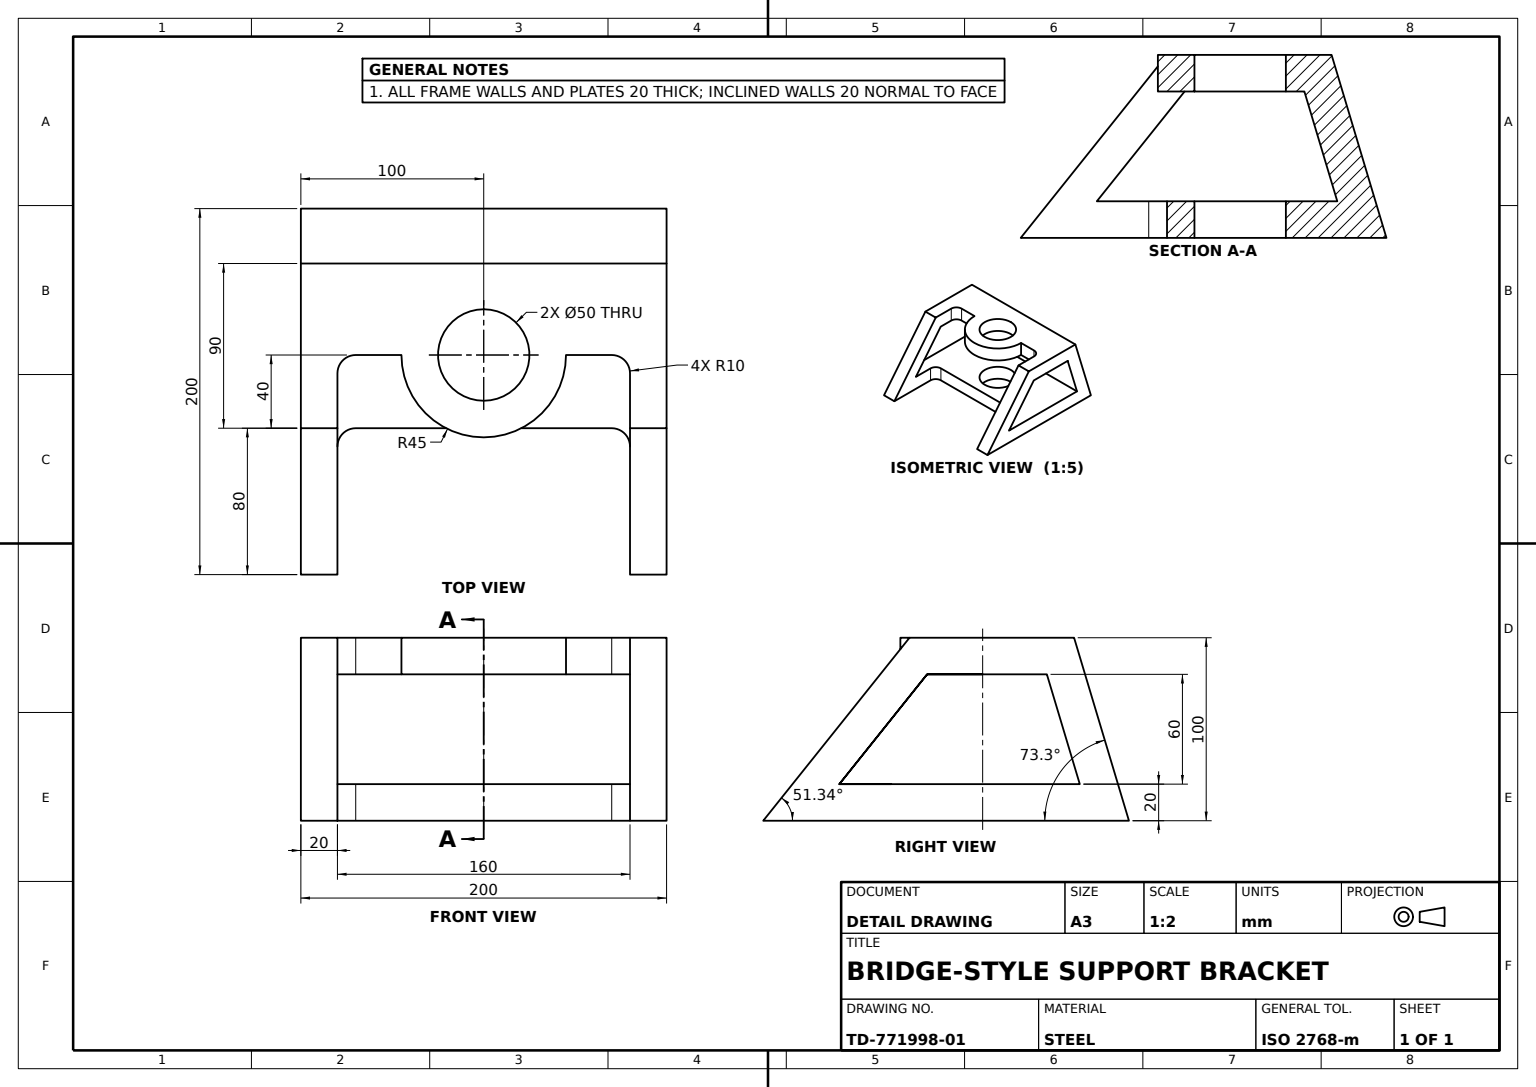
SolidWorks part; units mm, degrees
material "Plain Carbon Steel"
ref_plane "Front Plane" through (0, 0, 0) normal (0, 0, 1) x (1, 0, 0)
ref_plane "Top Plane" through (0, 0, 0) normal (0, 1, 0) x (1, 0, 0)
ref_plane "Right Plane" through (0, 0, 0) normal (1, 0, 0) x (0, 0, -1)
sketch "Frame Profile Sketch" plane through (0, 0, 0) normal (1, 0, 0) x (0, 0, -1)
  line L0 (200, 0) -> (170, 100)
  line L1 (170, 100) -> (80, 100)
  line L2 (80, 100) -> (0, 0)
  line L3 (0, 0) -> (200, 0)
  line L4 (155.1194, 80) -> (89.6125, 80)
  line L5 (89.6125, 80) -> (41.6125, 20)
  line L6 (41.6125, 20) -> (173.1194, 20)
  line L7 (173.1194, 20) -> (155.1194, 80)
  dimension "D1" = 30
  dimension "D2" = 90
  dimension "D3" = 80
  dimension "D5" = 60
  dimension "D4" = 20
extrude "Frame Body 200" add sketch "Frame Profile Sketch" along normal mid plane 200
sketch "Centre Recess Sketch" plane through (0, 0, 0) normal (0, 0, 1) x (1, 0, 0)
  line L1 (-80, 80) -> (80, 80)
  line L2 (-80, 80) -> (-80, 20)
  line L3 (-80, 20) -> (80, 20)
  line L4 (80, 80) -> (80, 20)
  line L5 (100, 0) -> (-100, 0) construction
  line L7 (0, 0) -> (0, 43.4052) construction
  point P4 (0, 80)
  point P8 (0, 20)
  dimension "D1" = 60
  dimension "D2" = 20
  dimension "D3" = 160
extrude "Centre Recess Cut" cut sketch "Centre Recess Sketch" against normal blind 150
sketch "Window A Sketch 80x60" plane through (0, 100, 0) normal (0, 1, 0) x (1, 0, 0)
  line L0 (80, 64) -> (80, 16) construction
  line L1 (-80, 120) -> (80, 120)
  line L2 (-80, 120) -> (-80, 60)
  line L3 (-80, 60) -> (80, 60)
  line L4 (80, 120) -> (80, 60)
  line L5 (-80, 16) -> (-80, 64) construction
  line L6 (100, 200) -> (-100, 200) construction
  dimension "D1" = 80
  dimension "D2" = 60
extrude "Window A Cut" cut sketch "Window A Sketch 80x60" against normal up to next
sketch "Window B Sketch" plane through (0, 20, 0) normal (0, 1, 0) x (1, 0, 0)
  line L0 (100, 0) -> (-100, 0) construction
  line L1 (-80, 0) -> (80, 0)
  line L2 (-80, 0) -> (-80, 80)
  line L3 (-80, 80) -> (80, 80)
  line L4 (80, 0) -> (80, 80)
  line L5 (-80, 41.6125) -> (-80, 16) construction
extrude "Window B Cut" cut sketch "Window B Sketch" against normal up to next
fillet "Window Corner Fillets R10" radius 10 4 edges at (-80, 10, -80) (-80, 90, -120) (80, 10, -80) (80, 90, -120)
sketch "Anchor Boss Sketch Ø90" plane through (0, 100, 0) normal (0, 1, 0) x (1, 0, 0)
  line L0 (70, 120) -> (-70, 120) construction
  circle A0 centre (0, 120) radius 45
  dimension "D1" = 90
extrude "Anchor Boss Ø90" add sketch "Anchor Boss Sketch Ø90" against normal up to surface (20 mm away) up to face at (0, 80, -113.2831)
sketch "Anchor Bore Sketch Ø50" plane through (0, 100, 0) normal (0, 1, 0) x (1, 0, 0)
  circle A0 centre (0, 120) radius 25
  arc A1 (-45, 120) -> (45, 120) centre (0, 120) ccw construction
  dimension "D1" = 50
extrude "Anchor Bore Ø50" cut sketch "Anchor Bore Sketch Ø50" against normal through all
